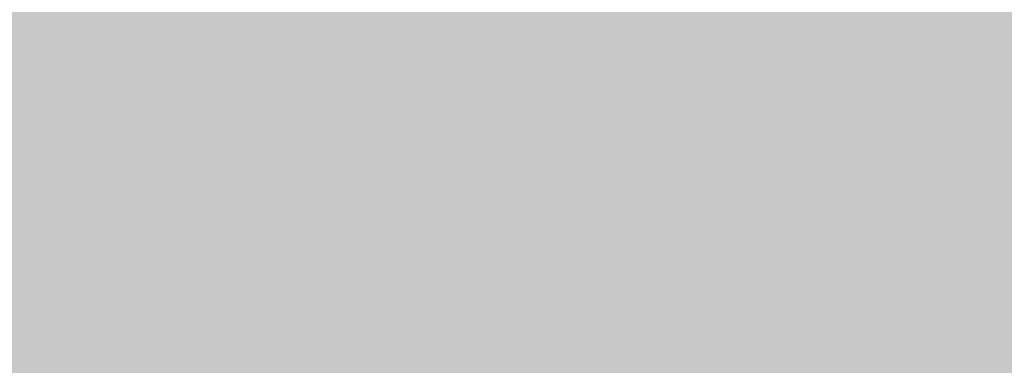
# Model space of a CAD drawing. Units: inches. Extents: x 2091 to 2899, y 967 to 2217.
# Tile 164 of 256: x 2203.144443 to 2203.14684, y 1152.2479 to 1152.248741. Entities that reach past the tile are written whole.
import ezdxf

# ---------------------------------------------------------------- set-up
doc = ezdxf.new("R2010")
doc.units = ezdxf.units.IN
doc.layers.add('A-WALL-PATT', color=141, linetype='Continuous', lineweight=13, true_color=0xadddf7)

msp = doc.modelspace()

# ---------------------------------------------------------------- hatches: boundary and pattern name
at = {"layer": 'A-WALL-PATT'}
h = msp.add_hatch(color=256, dxfattribs=at)
h.dxf.hatch_style = 1
h.paths.add_polyline_path([(2803.1436027, 2050.9190588), (2203.1436027, 2050.9190588), (2203.1436027, 1090.9190588), (2803.1436027, 1090.9190588)])
h.paths.add_polyline_path([(2635.7988501, 1147.5404649), (2674.5240524, 1147.5404649, 0.376086), (2678.5296653, 1152.8802017), (2678.5296653, 1159.5564734, 0.333335), (2674.524319, 1163.561846), (2674.524319, 1163.5618504), (2674.524319, 1192.9343904), (2635.8059707, 1192.9343904), (2597.0876225, 1192.9343904), (2597.0876225, 1163.561846, 0.333335), (2593.0822761, 1159.5564734), (2593.0822761, 1152.8802017, 0.376086), (2597.087889, 1147.5404649)], flags=0)
h.paths.add_polyline_path([(2436.0104329, 1278.2407784, 0.000483), (2435.9526433, 1278.215027, -0.001328), (2435.9356253, 1278.1116934, -0.001711), (2436.1164401, 1278.0407583, 0.002185)], flags=0)
h.paths.add_polyline_path([(2794.1436027, 1143.4190588), (2794.1436027, 1347.4190588), (2543.3701706, 1347.4190588), (2543.3701706, 1351.9190588), (2794.1436027, 1351.9190588), (2794.1436027, 1392.7135549), (2793.9473982, 1392.7135549), (2793.9473982, 1473.5368999), (2794.1436027, 1473.5368999), (2794.1436027, 1531.9190588), (2650.1436027, 1531.9190588), (2650.1436027, 1536.4190588), (2794.1436027, 1536.4190588), (2794.1436027, 1692.4190588), (2609.3756095, 1692.4190588), (2609.3756095, 1644.4190588), (2604.8756095, 1644.4190588), (2604.8756095, 1744.9190588), (2609.3756095, 1744.9190588), (2609.3756095, 1696.9190588), (2794.1436027, 1696.9190588), (2794.1436027, 1780.9190588), (2609.6436027, 1780.9190588), (2493.8756095, 1780.9190588), (2493.8756095, 1785.4190588), (2609.6436027, 1785.4190588), (2794.1436027, 1785.4190588), (2794.1436027, 1847.9388214), (2793.9512217, 1847.9388214), (2793.9512217, 1928.7621663), (2794.1436027, 1928.7621663), (2794.1436027, 1941.4190588), (2614.1436027, 1941.4190588), (2614.1436027, 1821.4190588), (2609.6436027, 1821.4190588), (2609.6436027, 1941.4190588), (2392.1436027, 1941.4190588), (2392.1436027, 1819.9190588), (2387.6436027, 1819.9190588), (2387.6436027, 1941.4190588), (2212.1436027, 1941.4190588), (2212.1436027, 1783.9190588), (2392.1436027, 1783.9190588), (2392.1436027, 1780.9190588), (2212.1436027, 1780.9190588), (2212.1436027, 1629.4190588), (2387.6436027, 1629.4190588), (2387.6436027, 1744.9190588), (2392.1436027, 1744.9190588), (2392.1436027, 1627.9190588), (2317.1436027, 1627.9190588), (2317.1436027, 1551.4190588), (2317.1436027, 1536.4190588), (2459.3835909, 1536.4190588), (2459.3835909, 1602.3964802), (2463.8835909, 1602.3964802), (2463.8835909, 1531.9190588), (2456.6436027, 1531.9190588), (2456.6436027, 1529.9190588), (2452.1436027, 1529.9190588), (2452.1436027, 1531.9190588), (2312.6436027, 1531.9190588), (2312.6436027, 1551.4190588), (2306.1436027, 1551.4190588), (2306.1436027, 1555.9190588), (2308.1436027, 1555.9190588), (2308.1436027, 1551.4190588), (2312.6436027, 1551.4190588), (2312.6436027, 1627.9190588), (2212.1436027, 1627.9190588), (2212.1436027, 1555.9190588), (2270.1436027, 1555.9190588), (2270.1436027, 1551.4190588), (2212.1436027, 1551.4190588), (2212.1436027, 1351.9190588), (2272.1436027, 1351.9190588), (2272.1436027, 1347.4190588), (2212.1436027, 1347.4190588), (2212.1436027, 1275.4190588), (2308.1436027, 1275.4190588), (2308.1436027, 1351.9190588), (2452.1436027, 1351.9190588), (2452.1436027, 1493.9190588), (2456.6436027, 1493.9190588), (2456.6436027, 1347.4190588), (2312.6436027, 1347.4190588), (2312.6436027, 1270.9190588), (2212.1436027, 1270.9190588), (2212.1436027, 1099.9190588), (2281.2375229, 1099.9190588), (2282.8710413, 1110.9138034), (2282.0083413, 1116.9966034), (2278.5577413, 1121.4204034), (2268.2056413, 1128.0562034), (2272.0876413, 1128.0562034), (2273.8129413, 1131.9270034), (2279.4203413, 1134.6919034), (2285.0278413, 1135.2449034), (2287.6158413, 1137.4568034), (2288.0471413, 1138.0098034), (2289.3411413, 1140.7747034), (2291.0665413, 1139.6687034), (2292.3605413, 1135.2449034), (2295.3798413, 1136.9038034), (2296.2425413, 1135.7979034), (2297.1052413, 1133.0330034), (2300.1246413, 1138.0098034), (2303.1439413, 1138.0098034), (2304.4379413, 1135.7979034), (2303.1439413, 1133.5860034), (2306.5946413, 1134.6919034), (2307.8887413, 1133.0330034), (2310.9080413, 1135.2449034), (2313.9274413, 1134.1389034), (2315.6268599, 1132.4271023), (2308.3200413, 1117.5496034), (2290.2038413, 1109.8079034), (2288.9098413, 1103.1721034), (2289.2723086, 1099.9190588), (2434.9182274, 1099.9190588), (2431.5932274, 1124.7880588), (2429.9302274, 1169.5530588), (2430.9271848, 1240.5196942), (2435.6589255, 1238.1861258), (2437.1352274, 1196.5540588), (2438.7982274, 1143.9730588), (2442.6782274, 1111.9980588), (2446.5582274, 1099.9190588), (2794.1436027, 1099.9190588), (2794.1436027, 1138.9190588), (2548.0324471, 1138.9190588), (2548.0324471, 1143.4190588), (2548.0324471, 1148.8190588), (2546.6684571, 1148.0315588), (2528.6856919, 1179.1786218, 0.256256), (2512.0324471, 1148.8190588), (2512.0324471, 1143.4190588), (2512.0324471, 1138.9190588), (2507.5324471, 1138.9190588), (2507.5324471, 1143.4190588), (2507.5324471, 1148.8190588, 0.256256), (2490.8792023, 1179.1786218), (2472.8964371, 1148.0315588), (2471.5324471, 1148.8190588), (2471.5324471, 1143.4190588), (2467.0324471, 1143.4190588), (2467.0324471, 1269.9457858, 0.039061), (2460.9099871, 1273.5800588), (2467.0324471, 1273.5800588), (2467.0324471, 1286.3253638, 0.014511), (2465.2161944, 1286.7619052), (2467.0324471, 1287.0525761), (2467.0324471, 1323.4190588), (2471.5324471, 1323.4190588), (2471.5324471, 1148.8190588), (2489.5324471, 1179.9959734), (2490.8964371, 1179.2084734), (2490.8792023, 1179.1786218, -0.256256), (2507.5324471, 1148.8190588), (2507.5324471, 1143.4190588), (2512.0324471, 1143.4190588), (2512.0324471, 1148.8190588, -0.256256), (2528.6856919, 1179.1786218), (2528.6684571, 1179.2084734), (2530.0324471, 1179.9959734), (2548.0324471, 1148.8190588), (2548.0324471, 1143.4190588)], flags=16)
h.paths.add_polyline_path([(2607.7685461, 1200.9450832), (2607.7685461, 1265.0306251), (2597.0876225, 1281.0520106), (2619.7845852, 1281.0520106), (2627.795278, 1337.1268598), (2635.7988501, 1337.1268598), (2643.8166634, 1337.1268598), (2651.8273562, 1281.0520106), (2674.524319, 1281.0520106), (2663.8433953, 1265.0306251), (2663.8433953, 1200.9450832), (2635.8059707, 1200.9450832)], flags=0)
edge = h.paths.add_edge_path(flags=0)
edge.add_ellipse((13303.8962153, 1272.9987247), major_axis=(-10595.3130399, 0.0000005), ratio=0.842303870086, start_angle=0.62823721906, end_angle=0.64655409989, ccw=False)
edge.add_ellipse((2711.7004495, 1156.8526781), major_axis=(2.2197691, 0), ratio=0.84230387, start_angle=111.5352435, end_angle=180.6282372, ccw=False)
edge.add_ellipse((13303.1562922, 1272.9987246), major_axis=(-10593.0263064, 0), ratio=0.842303869544, start_angle=0.52827147182, end_angle=0.64655409706, ccw=False)
edge.add_line((2710.7645961, 1175.3332951), (2710.1299858, 1175.3332951))
edge.add_ellipse((2710.1299858, 1176.5797752), major_axis=(1.4798461, 0), ratio=0.84230387, start_angle=180, end_angle=270, ccw=False)
edge.add_line((2708.6501397, 1176.5797752), (2708.6501397, 1200.7829144))
edge.add_ellipse((2710.1299858, 1200.7829144), major_axis=(1.4798461, 0), ratio=0.84230387, start_angle=90, end_angle=180, ccw=False)
edge.add_line((2710.1299858, 1202.0293944), (2710.4650752, 1202.0293944))
edge.add_ellipse((13303.1562922, 1272.9987246), major_axis=(-10593.0263064, 0), ratio=0.842303869544, start_angle=-0.09022908859, end_angle=0.38386677879, ccw=False)
edge.add_ellipse((2710.1299858, 1290.9270308), major_axis=(-1.4798461, 0), ratio=0.84230387, start_angle=0, end_angle=90, ccw=False)
edge.add_line((2708.6501397, 1290.9270308), (2708.6501397, 1315.13017))
edge.add_ellipse((2710.1299858, 1315.13017), major_axis=(-1.4798461, 0), ratio=0.84230387, start_angle=-90, end_angle=0, ccw=False)
edge.add_line((2710.1299858, 1316.3766501), (2710.7063141, 1316.3766501))
edge.add_ellipse((3238.4017202, 1296.2895655), major_axis=(528.2339998, 0), ratio=0.84230386954, start_angle=176.349572414, end_angle=177.820049686, ccw=False)
edge.add_ellipse((2775.0630432, 1071.4506962), major_axis=(313.3077613, 0), ratio=0.84230386954, start_angle=102.125965552, end_angle=103.780528989, ccw=False)
edge.add_ellipse((2775.0630432, 1078.3056979), major_axis=(-305.3028915, 0), ratio=0.84230386955, start_angle=-79.790461003, end_angle=-77.555372706, ccw=False)
edge.add_ellipse((2695.1417666, 1541.9753825), major_axis=(-250.9602162, 0), ratio=0.84230386954, start_angle=99.256566007, end_angle=102.554932644)
edge.add_line((2741.4103262, 1334.2142554), (2747.1325454, 1337.3784768))
edge.add_ellipse((2747.5386163, 1336.8574776), major_axis=(-0.739923, 0), ratio=0.84230387, start_angle=270, end_angle=307.9331305, ccw=False)
edge.add_ellipse((2747.5386163, 1336.8574776), major_axis=(-0.739923, 0), ratio=0.84230387, start_angle=232.0668695, end_angle=270, ccw=False)
edge.add_line((2747.9446872, 1337.3784768), (2753.6669064, 1334.2142554))
edge.add_ellipse((2799.935466, 1541.9753825), major_axis=(250.9602162, 0), ratio=0.84230386954, start_angle=257.445067356, end_angle=260.743433993)
edge.add_ellipse((2720.0141894, 1078.3056979), major_axis=(305.3028915, 0), ratio=0.84230386954, start_angle=77.555372707, end_angle=79.790461003, ccw=False)
edge.add_ellipse((2720.0141894, 1071.4506962), major_axis=(-313.3077613, 0), ratio=0.84230386954, start_angle=256.219471011, end_angle=257.874034448, ccw=False)
edge.add_ellipse((2256.6755124, 1296.2895655), major_axis=(-528.2339998, 0), ratio=0.84230386954, start_angle=182.179950314, end_angle=183.650427586, ccw=False)
edge.add_line((2784.3709184, 1316.3766501), (2784.9472468, 1316.3766501))
edge.add_ellipse((2784.9472468, 1315.13017), major_axis=(1.4798461, 0), ratio=0.84230387, start_angle=0, end_angle=90, ccw=False)
edge.add_line((2786.4270928, 1315.13017), (2786.4270928, 1290.9270308))
edge.add_ellipse((2784.9472468, 1290.9270308), major_axis=(1.4798461, 0), ratio=0.84230387, start_angle=270, end_angle=360, ccw=False)
edge.add_ellipse((-7808.0790596, 1272.9987246), major_axis=(10593.0263063, 0), ratio=0.842303869544, start_angle=-0.38386677879, end_angle=0.09022908859, ccw=False)
edge.add_line((2784.6121574, 1202.0293944), (2784.9472468, 1202.0293944))
edge.add_ellipse((2784.9472468, 1200.7829144), major_axis=(1.4798461, 0), ratio=0.84230387, start_angle=0, end_angle=90, ccw=False)
edge.add_line((2786.4270928, 1200.7829144), (2786.4270928, 1176.5797752))
edge.add_ellipse((2784.9472468, 1176.5797752), major_axis=(-1.4798461, 0), ratio=0.84230387, start_angle=90, end_angle=180, ccw=False)
edge.add_line((2784.9472468, 1175.3332951), (2784.3126365, 1175.3332951))
edge.add_ellipse((-7808.0790596, 1272.9987246), major_axis=(10593.0263063, 0), ratio=0.842303869544, start_angle=-0.61864319632, end_angle=-0.52827147182, ccw=False)
edge.add_ellipse((2783.3767831, 1156.8526781), major_axis=(-2.2197691, 0), ratio=0.84230387, start_angle=179.3717628, end_angle=248.4647566, ccw=False)
edge.add_ellipse((-7808.8189826, 1272.9987246), major_axis=(-10595.3130398, 0.0000036), ratio=0.842303865762, start_angle=179.3534459226, end_angle=179.37176280343, ccw=False)
edge.add_ellipse((2780.2973026, 1153.500793), major_axis=(-5.2464256, 0), ratio=0.84230387, start_angle=90, end_angle=179.3534459, ccw=False)
edge.add_line((2780.2973026, 1149.0817084), (2714.77993, 1149.0817084))
edge.add_ellipse((2714.77993, 1153.500793), major_axis=(5.2464256, 0), ratio=0.84230387, start_angle=180.6465541, end_angle=270, ccw=False)
edge = h.paths.add_edge_path(flags=0)
edge.add_line((2718.1873674, 1151.0078329), (2718.1873674, 1170.4723638))
edge.add_ellipse((2721.1470595, 1170.4723638), major_axis=(-2.9596921, 0), ratio=0.84230387, start_angle=-90, end_angle=0, ccw=False)
edge.add_line((2721.1470595, 1172.965324), (2773.9301731, 1172.965324))
edge.add_ellipse((2773.9301731, 1170.4723638), major_axis=(-2.9596921, 0), ratio=0.84230387, start_angle=180, end_angle=270, ccw=False)
edge.add_line((2776.8898652, 1170.4723638), (2776.8898652, 1151.0078329))
edge.add_line((2776.8898652, 1151.0078329), (2718.1873674, 1151.0078329))
edge = h.paths.add_edge_path(flags=0)
edge.add_line((2718.1873674, 1180.2341502), (2718.1873674, 1199.0578342))
edge.add_ellipse((2747.5386163, 1320.3986402), major_axis=(147.0179239, 0), ratio=0.84230386954, start_angle=256.40186531, end_angle=283.59813469)
edge.add_line((2776.8898652, 1199.0578342), (2776.8898652, 1180.2341502))
edge.add_ellipse((2747.5386163, 1301.5749562), major_axis=(147.0179239, 0), ratio=0.84230386954, start_angle=256.40186531, end_angle=283.59813469, ccw=False)
edge = h.paths.add_edge_path(flags=0)
edge.add_ellipse((13303.1562922, 1272.9987246), major_axis=(-10591.5464603, 0), ratio=0.842303869555, start_angle=0.05559431352, end_angle=0.37776419393, ccw=False)
edge.add_line((2711.6168595, 1262.7217103), (2715.6674076, 1249.4953957))
edge.add_ellipse((6413.8919626, 1241.691919), major_axis=(-3698.2361592, 0), ratio=0.842303869547, start_angle=-0.120897369, end_angle=0.3640763489)
edge.add_line((2715.7610383, 1218.1924547), (2711.9343065, 1203.167361))
edge = h.paths.add_edge_path(flags=0)
edge.add_line((2718.1873674, 1251.074566), (2716.0024854, 1267.4504351))
edge.add_ellipse((2742.1511746, 1202.1895399), major_axis=(81.7725845, 0), ratio=0.8423038695, start_angle=94.277420963, end_angle=111.834953797, ccw=False)
edge.add_line((2737.0097482, 1270.9306255), (2758.0674844, 1270.9306255))
edge.add_ellipse((2752.926058, 1202.1895399), major_axis=(81.7725845, 0), ratio=0.8423038695, start_angle=68.165046203, end_angle=85.722579037, ccw=False)
edge.add_line((2779.0747472, 1267.4504351), (2776.8898652, 1251.074566))
edge.add_ellipse((2750.3380588, 1187.8853558), major_axis=(79.5796641, 0), ratio=0.8423038695, start_angle=67.208085122, end_angle=85.129930403)
edge.add_line((2756.0346562, 1254.7436557), (2739.0425764, 1254.7436557))
edge.add_ellipse((2744.7391738, 1187.8853558), major_axis=(79.5796641, 0), ratio=0.8423038695, start_angle=94.870069597, end_angle=112.791914878)
edge = h.paths.add_edge_path(flags=0)
edge.add_line((2783.1429261, 1203.167361), (2779.3161943, 1218.1924547))
edge.add_ellipse((-918.81473, 1241.691919), major_axis=(3698.2361592, 0), ratio=0.842303869546, start_angle=-0.3640763489, end_angle=0.120897369)
edge.add_line((2779.409825, 1249.4953957), (2783.4603731, 1262.7217103))
edge.add_ellipse((-7808.0790596, 1272.9987246), major_axis=(-10591.5464603, 0), ratio=0.84230386954, start_angle=179.6222358061, end_angle=179.94440568651, ccw=False)
edge = h.paths.add_edge_path(flags=0)
edge.add_ellipse((2734.2008921, 1286.6904402), major_axis=(-0.3566086, 6.3400775), ratio=0.603833576, start_angle=89.00201428, end_angle=253.65740805, ccw=False)
edge.add_line((2730.3690013, 1286.5418057), (2730.3690013, 1301.3519803))
edge.add_line((2730.3690013, 1301.3519803), (2735.9133107, 1305.2148028))
edge.add_ellipse((2736.3849168, 1304.7345612), major_axis=(0.739923, 0), ratio=0.84230387, start_angle=90, end_angle=134.4802109, ccw=False)
edge.add_line((2736.3849168, 1305.3578013), (2738.0327829, 1305.3578013))
edge.add_line((2738.0327829, 1305.3578013), (2738.0327829, 1307.7079274))
edge.add_ellipse((2794.201642, 1307.7079274), major_axis=(56.168859, 0), ratio=0.8423038695, start_angle=150.5614304, end_angle=180, ccw=False)
edge.add_ellipse((2700.8755906, 1307.7079274), major_axis=(-56.168859, 0), ratio=0.8423038695, start_angle=180, end_angle=209.4385696, ccw=False)
edge.add_line((2757.0444497, 1307.7079274), (2757.0444497, 1305.3578013))
edge.add_line((2757.0444497, 1305.3578013), (2758.6923157, 1305.3578013))
edge.add_ellipse((2758.6923157, 1304.7345612), major_axis=(-0.739923, 0), ratio=0.84230387, start_angle=225.5197891, end_angle=270, ccw=False)
edge.add_line((2759.1639219, 1305.2148028), (2764.7082312, 1301.3519803))
edge.add_line((2764.7082312, 1301.3519803), (2764.7082312, 1286.5418057))
edge.add_ellipse((2760.8763405, 1286.6904402), major_axis=(0.3566086, 6.3400775), ratio=0.603833576, start_angle=106.34259195, end_angle=270.99798572, ccw=False)
edge.add_line((2757.0444497, 1285.7970896), (2757.0444497, 1307.7079274))
edge.add_ellipse((2700.8755906, 1307.7079274), major_axis=(-56.168859, 0), ratio=0.8423038695, start_angle=180, end_angle=209.4385696)
edge.add_ellipse((2794.201642, 1307.7079274), major_axis=(56.168859, 0), ratio=0.8423038695, start_angle=150.5614304, end_angle=180)
edge.add_line((2738.0327829, 1307.7079274), (2738.0327829, 1285.7970896))
h.paths.add_polyline_path([(2417.8122727, 1104.449704), (2413.4922727, 1102.529704), (2410.6122727, 1103.969704), (2409.1722727, 1106.369704), (2407.2522727, 1107.329704), (2406.2922727, 1109.729704), (2405.3322727, 1114.049704), (2405.3322727, 1117.889704), (2406.2922727, 1120.129704), (2407.2522727, 1119.809704), (2408.8483218, 1118.3276585), (2410.1739451, 1119.4241703), (2410.2112727, 1120.405704), (2411.0407305, 1121.4190541), (2410.6992727, 1119.858704), (2410.1739451, 1119.4241703), (2410.0884515, 1117.1761095), (2411.1328361, 1116.2063237), (2413.9722727, 1119.329704), (2416.8522727, 1120.769704), (2416.8697209, 1120.7987842), (2417.0350713, 1119.4051162), (2417.8962134, 1118.1433844), (2418.2922727, 1118.369704), (2419.5444467, 1120.0392692), (2419.3609153, 1118.387487), (2419.0321078, 1119.3561507), (2418.3989394, 1118.5119262), (2419.2522727, 1114.529704), (2418.7940909, 1107.1987949)], flags=0)
h.paths.add_polyline_path([(2508.8701706, 1347.4190588), (2508.3701706, 1347.4190588), (2508.3701706, 1351.9190588), (2508.8701706, 1351.9190588)], flags=0)
h.paths.add_polyline_path([(2473.3701706, 1347.4190588), (2472.3701706, 1347.4190588), (2467.8701706, 1347.4190588), (2467.8701706, 1455.4190588), (2472.3701706, 1455.4190588), (2472.3701706, 1352.4190588), (2473.3701706, 1352.4190588)], flags=0)
h.paths.add_polyline_path([(2352.106244, 1217.4461971), (2349.226244, 1218.8861971), (2347.786244, 1221.2861971), (2345.866244, 1222.2461971), (2344.906244, 1224.6461971), (2343.946244, 1228.9661971), (2343.946244, 1232.8061971), (2344.906244, 1235.0461971), (2345.866244, 1234.7261971), (2347.4622931, 1233.2441515), (2348.7879164, 1234.3406634), (2348.825244, 1235.3221971), (2349.6547018, 1236.3355471), (2349.313244, 1234.7751971), (2348.7879164, 1234.3406634), (2348.7024228, 1232.0926025), (2349.7468074, 1231.1228168), (2352.586244, 1234.2461971), (2355.466244, 1235.6861971), (2355.4836921, 1235.7152773), (2355.6490426, 1234.3216093), (2356.5101846, 1233.0598774), (2356.906244, 1233.2861971), (2358.1584179, 1234.9557623), (2357.9748866, 1233.3039801), (2357.6460791, 1234.2726438), (2357.0129107, 1233.4284193), (2357.866244, 1229.4461971), (2357.4080622, 1222.115288), (2356.426244, 1219.3661971)], flags=0)
h.paths.add_polyline_path([(2348.2967999, 1112.2244204), (2347.0137999, 1112.3104204), (2345.5297999, 1114.1274204), (2345.7317999, 1115.8584204), (2346.8117999, 1116.9824204), (2346.8117999, 1114.6464204), (2345.8667999, 1114.2144204), (2346.8797999, 1114.3004204)], flags=0)
h.paths.add_polyline_path([(2347.0137999, 1110.9264204), (2346.2717999, 1110.4934204), (2346.6097999, 1111.1864204)], flags=0)
h.paths.add_polyline_path([(2345.8667999, 1118.1944204), (2345.5297999, 1117.3294204), (2343.7077999, 1118.0214204), (2344.3827999, 1118.6264204)], flags=0)
h.paths.add_polyline_path([(2346.6767999, 1109.2824204), (2346.0697999, 1108.0714204), (2345.8667999, 1110.0614204)], flags=0)
h.paths.add_polyline_path([(2345.0567999, 1119.7514204), (2343.6397999, 1119.7514204), (2343.9777999, 1121.1354204)], flags=0)
h.paths.add_polyline_path([(2345.2597999, 1116.5504204), (2345.1247999, 1115.8584204), (2344.9217999, 1115.6854204), (2344.7197999, 1116.3774204)], flags=0)
h.paths.add_polyline_path([(2345.6647999, 1112.3104204), (2345.4617999, 1111.5324204), (2344.0447999, 1111.9644204), (2344.6517999, 1112.5704204)], flags=0)
h.paths.add_polyline_path([(2345.1917999, 1113.3494204), (2344.4497999, 1113.8684204), (2344.7197999, 1114.3874204)], flags=0)
h.paths.add_polyline_path([(2344.6517999, 1116.8094204), (2344.1797999, 1115.6854204), (2344.6517999, 1115.3394204), (2343.9097999, 1114.9064204), (2343.0327999, 1115.9444204), (2343.6397999, 1116.4634204)], flags=0)
h.paths.add_polyline_path([(2345.8667999, 1106.6864204), (2344.9897999, 1105.5624204), (2344.5167999, 1106.6004204)], flags=0)
h.paths.add_polyline_path([(2344.8547999, 1110.0614204), (2344.5167999, 1109.2824204), (2344.1127999, 1109.7154204)], flags=0)
h.paths.add_polyline_path([(2344.0447999, 1113.5224204), (2343.4377999, 1113.0894204), (2342.7627999, 1113.9544204)], flags=0)
h.paths.add_polyline_path([(2344.3147999, 1111.0124204), (2342.9647999, 1110.3204204), (2342.9647999, 1111.0994204)], flags=0)
h.paths.add_polyline_path([(2345.1247999, 1104.6974204), (2344.5847999, 1103.7454204), (2344.4497999, 1104.2644204)], flags=0)
h.paths.add_polyline_path([(2342.8297999, 1121.2224204), (2341.7497999, 1120.5304204), (2340.5357999, 1121.0494204), (2340.1307999, 1121.8284204), (2340.6707999, 1122.9524204), (2341.1427999, 1121.8284204), (2341.6147999, 1122.0014204)], flags=0)
h.paths.add_polyline_path([(2342.9647999, 1119.7514204), (2343.0327999, 1118.4534204), (2342.0877999, 1118.0214204), (2342.0197999, 1119.4914204)], flags=0)
h.paths.add_polyline_path([(2342.6947999, 1116.8964204), (2341.9527999, 1116.6364204), (2342.0197999, 1117.3294204)], flags=0)
h.paths.add_polyline_path([(2343.0327999, 1112.2244204), (2342.0197999, 1111.7914204), (2341.5477999, 1112.2244204), (2342.3577999, 1113.3494204)], flags=0)
h.paths.add_polyline_path([(2343.7747999, 1104.4374204), (2342.6277999, 1102.8804204), (2342.6947999, 1104.6104204), (2343.4377999, 1105.1294204)], flags=0)
h.paths.add_polyline_path([(2342.0197999, 1115.0794204), (2340.8057999, 1115.5124204), (2340.9407999, 1116.3774204)], flags=0)
h.paths.add_polyline_path([(2341.4807999, 1120.0974204), (2341.4807999, 1119.4054204), (2341.0757999, 1119.5784204), (2341.1427999, 1120.0974204)], flags=0)
h.paths.add_polyline_path([(2341.8177999, 1114.4734204), (2340.9407999, 1113.0894204), (2340.8057999, 1114.5604204)], flags=0)
h.paths.add_polyline_path([(2341.1427999, 1118.5404204), (2340.9407999, 1116.9824204), (2339.0507999, 1117.6754204), (2339.0507999, 1118.6264204)], flags=0)
h.paths.add_polyline_path([(2342.6947999, 1101.6684204), (2341.9527999, 1101.8414204), (2342.5597999, 1102.3614204)], flags=0)
h.paths.add_polyline_path([(2340.3327999, 1119.6654204), (2338.4437999, 1119.5784204), (2337.9037999, 1120.3574204), (2339.6577999, 1120.6164204)], flags=0)
h.paths.add_polyline_path([(2340.3327999, 1115.3394204), (2340.0627999, 1113.6954204), (2339.3877999, 1115.3394204)], flags=0)
h.paths.add_polyline_path([(2341.8177999, 1103.8314204), (2341.5477999, 1102.8804204), (2341.1427999, 1103.6584204)], flags=0)
h.paths.add_polyline_path([(2339.0507999, 1122.8664204), (2337.2957999, 1121.8284204), (2337.0937999, 1123.1254204), (2337.7687999, 1123.8184204)], flags=0)
h.paths.add_polyline_path([(2339.1177999, 1121.7414204), (2338.8477999, 1121.2224204), (2338.1737999, 1121.0494204), (2338.3757999, 1121.5684204)], flags=0)
h.paths.add_polyline_path([(2339.1857999, 1119.3194204), (2338.6457999, 1118.7134204), (2338.2407999, 1118.1074204), (2338.2407999, 1118.8864204)], flags=0)
h.paths.add_polyline_path([(2341.1427999, 1101.9284204), (2340.6027999, 1101.2364204), (2340.0627999, 1101.8414204), (2340.6027999, 1102.3614204)], flags=0)
h.paths.add_polyline_path([(2337.6337999, 1117.7614204), (2336.6207999, 1118.2804204), (2337.2957999, 1118.9724204)], flags=0)
h.paths.add_polyline_path([(2336.8237999, 1119.5784204), (2334.7987999, 1118.9724204), (2335.2037999, 1120.3574204), (2336.5537999, 1120.8764204)], flags=0)
h.paths.add_polyline_path([(2339.1177999, 1100.4574204), (2337.3637999, 1100.5434204), (2336.7557999, 1101.2364204)], flags=0)
h.paths.add_polyline_path([(2336.3507999, 1122.4334204), (2336.0137999, 1121.9144204), (2334.9337999, 1122.4334204), (2334.5287999, 1123.4714204), (2335.7437999, 1122.7794204)], flags=0)
h.paths.add_polyline_path([(2334.7317999, 1120.8764204), (2334.2587999, 1120.3574204), (2334.0567999, 1120.7894204), (2334.5967999, 1121.3084204)], flags=0)
h.paths.add_polyline_path([(2334.4617999, 1122.1744204), (2332.5717999, 1121.3084204), (2331.3567999, 1122.1744204), (2332.0997999, 1122.8664204)], flags=0)
h.paths.add_polyline_path([(2334.2587999, 1118.5404204), (2333.3817999, 1118.4534204), (2333.6517999, 1119.3194204)], flags=0)
h.paths.add_polyline_path([(2335.5417999, 1102.2744204), (2334.1917999, 1102.6204204), (2335.2717999, 1103.3124204)], flags=0)
h.paths.add_polyline_path([(2332.7067999, 1119.6654204), (2331.6947999, 1120.4434204), (2332.5047999, 1120.7894204)], flags=0)
h.paths.add_polyline_path([(2334.7317999, 1101.1494204), (2333.5167999, 1101.5824204), (2333.9887999, 1101.7554204)], flags=0)
h.paths.add_polyline_path([(2332.6397999, 1116.6364204), (2331.0867999, 1116.2904204), (2331.9647999, 1118.1944204)], flags=0)
h.paths.add_polyline_path([(2330.7497999, 1121.5684204), (2330.2767999, 1120.2704204), (2328.5227999, 1119.3194204), (2328.9947999, 1121.0494204)], flags=0)
h.paths.add_polyline_path([(2330.7497999, 1118.6264204), (2330.0077999, 1117.5024204), (2329.8727999, 1118.0214204)], flags=0)
h.paths.add_polyline_path([(2332.0997999, 1102.3614204), (2330.5467999, 1102.0144204), (2331.6947999, 1102.9664204)], flags=0)
h.paths.add_polyline_path([(2329.5347999, 1113.6084204), (2329.0627999, 1112.3104204), (2328.5897999, 1113.3494204)], flags=0)
h.paths.add_polyline_path([(2328.3877999, 1117.8484204), (2327.5097999, 1116.5504204), (2327.1727999, 1117.7614204)], flags=0)
h.paths.add_polyline_path([(2329.7377999, 1106.5134204), (2329.5347999, 1105.3024204), (2328.2527999, 1106.0814204)], flags=0)
h.paths.add_polyline_path([(2328.6577999, 1114.3874204), (2328.0497999, 1114.1274204), (2328.3197999, 1114.9064204)], flags=0)
h.paths.add_polyline_path([(2328.3197999, 1112.2244204), (2327.1057999, 1112.1374204), (2326.7007999, 1112.6564204)], flags=0)
h.paths.add_polyline_path([(2326.9027999, 1115.2524204), (2326.7007999, 1114.1274204), (2325.2157999, 1113.6084204), (2326.0927999, 1115.3394204)], flags=0)
h.paths.add_polyline_path([(2326.6327999, 1108.3304204), (2326.0927999, 1107.3794204), (2325.8907999, 1108.5034204), (2326.4977999, 1109.1094204)], flags=0)
h.paths.add_polyline_path([(2615.1436027, 1531.9190588), (2609.6436027, 1531.9190588), (2609.6436027, 1620.4190588), (2614.1436027, 1620.4190588), (2614.1436027, 1536.4190588), (2615.1436027, 1536.4190588)], flags=0)
h.paths.add_polyline_path([(2545.1436027, 1563.4190588), (2464.1436027, 1563.4190588), (2464.1436027, 1632.4190588), (2509.1436027, 1632.4190588), (2509.1436027, 1627.9190588), (2509.1436027, 1603.9190588), (2468.6436027, 1603.9190588), (2468.6436027, 1567.9190588), (2540.6436027, 1567.9190588), (2540.6436027, 1591.9190588), (2545.1436027, 1591.9190588)], flags=0)
h.paths.add_polyline_path([(2388.9690483, 1549.985735), (2357.4341811, 1549.985735), (2357.4341811, 1623.3607783), (2399.3627772, 1623.3607783), (2435.6894654, 1623.3607783), (2435.5925469, 1602.5592734), (2435.5925469, 1602.3964802), (2388.9690483, 1602.3964802)], flags=0)
h.paths.add_polyline_path([(2388.8806282, 1555.8091511), (2374.9044295, 1555.8091511), (2374.9044295, 1600.5715641), (2374.9044295, 1615.4576454), (2406.3508766, 1615.4576454), (2406.3508766, 1618.9394309), (2412.1742927, 1615.4576454), (2406.3508766, 1611.9758599), (2406.3508766, 1615.4576454), (2388.8806282, 1615.4576454)], flags=0)
h.paths.add_polyline_path([(2568.8756095, 1644.4190588), (2453.3756095, 1644.4190588), (2453.3756095, 1785.4190588), (2457.8756095, 1785.4190588), (2457.8756095, 1648.9190588), (2568.8756095, 1648.9190588)], flags=0)
h.paths.add_polyline_path([(2212.1436027, 1945.9190588), (2212.1436027, 2041.9190588), (2794.1436027, 2041.9190588), (2794.1436027, 1945.9190588)], flags=16)
h.paths.add_polyline_path([(2271.0827276, 1964.3172377), (2776.852968, 1964.3172377), (2776.852968, 2037.1696226), (2271.0827276, 2037.1696226)], flags=8)
h.paths.add_polyline_path([(2380.6492852, 1536.8241435), (2461.0408087, 1536.8241435), (2461.0408087, 1554.6525871), (2380.6492852, 1554.6525871)], flags=8)
h.paths.add_polyline_path([(2240.7557092, 1609.7254508), (2309.1858294, 1609.7254508), (2309.1858294, 1617.6982037), (2240.7557092, 1617.6982037)], flags=8)
h.paths.add_polyline_path([(2212.6772554, 1313.5041021), (2282.5915203, 1313.5041021), (2282.5915203, 1322.7452389), (2212.6772554, 1322.7452389)], flags=8)
h.paths.add_polyline_path([(2457.111976, 1114.778574), (2558.4815807, 1114.778574), (2558.4815807, 1142.2196823), (2457.111976, 1142.2196823)], flags=8)
h.paths.add_polyline_path([(2473.4423372, 1273.0100672), (2604.6412257, 1273.0100672), (2604.6412257, 1318.3469349), (2473.4423372, 1318.3469349)], flags=8)
h.paths.add_polyline_path([(2638.8763024, 1626.9774316), (2684.2503675, 1627.9767377), (2684.0384825, 1637.5974944), (2638.6644174, 1636.5981884)], flags=8)
h.paths.add_polyline_path([(2537.5905538, 1453.7934466), (2628.3895472, 1453.7934466), (2628.3895472, 1475.3448114), (2537.5905538, 1475.3448114)], flags=8)
h.paths.add_polyline_path([(2504.1376376, 1714.6323972), (2554.6471875, 1714.6323972), (2554.6471875, 1730.2377115), (2504.1376376, 1730.2377115)], flags=8)
h.paths.add_polyline_path([(2487.5011806, 1575.6518716), (2535.0971214, 1575.6518716), (2535.0971214, 1598.3776456), (2487.5011806, 1598.3776456)], flags=8)
h.paths.add_polyline_path([(2709.0994004, 1735.7102784), (2740.0166009, 1735.7102784), (2740.0166009, 1749.9376406), (2709.0994004, 1749.9376406)], flags=8)
h.paths.add_polyline_path([(2442.4384239, 1792.1716575), (2564.7288353, 1792.1716575), (2564.7288353, 1842.0001626), (2442.4384239, 1842.0001626)], flags=8)
h.paths.add_polyline_path([(2655.8158012, 1809.6440763), (2789.5201425, 1806.6937963), (2790.0849768, 1832.2916379), (2656.3806355, 1835.2419179)], flags=8)
h.paths.add_polyline_path([(2234.8426972, 1797.7201432), (2368.5928512, 1794.7688523), (2369.1607182, 1820.504132), (2235.4105642, 1823.4554229)], flags=8)
h.paths.add_polyline_path([(2245.1384659, 1644.0063348), (2398.4277329, 1640.6238997), (2398.9948417, 1666.3248199), (2245.7055747, 1669.7072549)], flags=8)
h.paths.add_polyline_path([(2306.1428474, 1431.1685186), (2413.7683138, 1428.7936873), (2414.3331481, 1454.3915289), (2306.7076817, 1456.7663602)], flags=8)
h.paths.add_polyline_path([(2306.834582, 1458.2331447), (2393.3804836, 1456.3234487), (2393.9328082, 1481.3543583), (2307.3869066, 1483.2640542)], flags=8)

doc.saveas('drawing.dxf')
